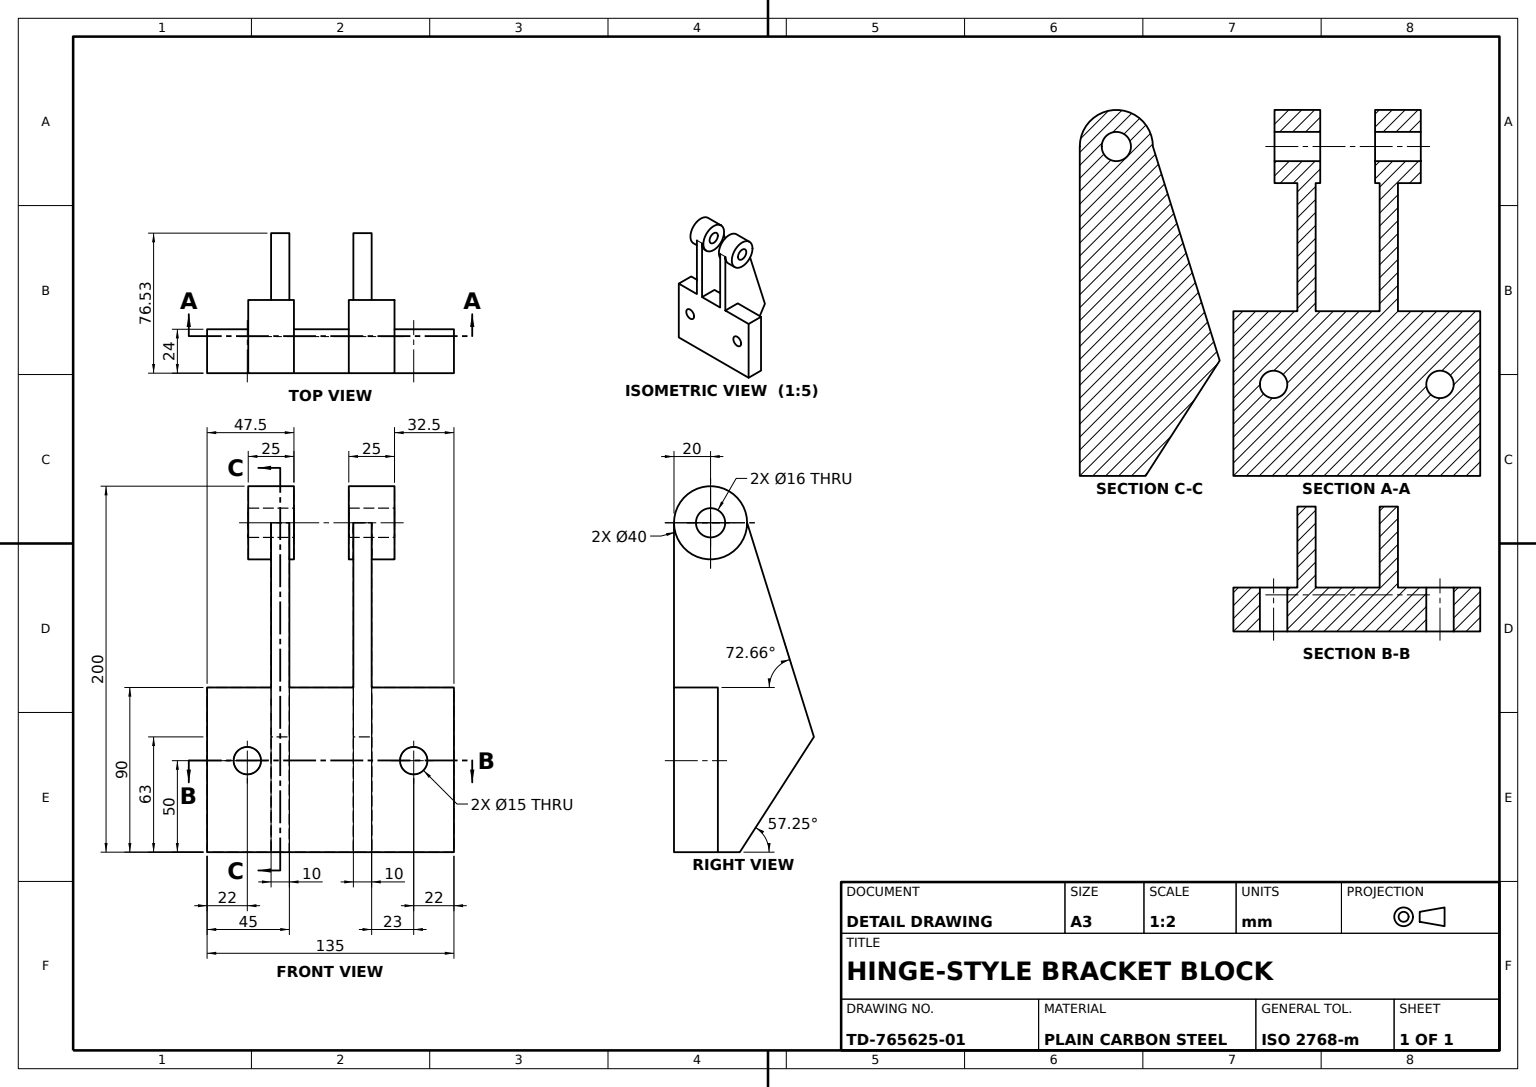
from build123d import *

# Parameters (mm, degrees)
BASE_PLATE_SKETCH_W     = 135
BASE_PLATE_SKETCH_H     = 90
BASE_PLATE_DEPTH        = 24
LUG_1_DEPTH             = 10
LUG_1_BOSS_SKETCH_R     = 20
LUG_1_PIVOT_BOSS_DEPTH  = 12.5
LUG_2_DEPTH             = 10
LUG_2_BOSS_SKETCH_R     = 20
LUG_2_PIVOT_BOSS_DEPTH  = 12.5
PIVOT_HOLE_SKETCH_R     = 8
PIVOT_HOLE_16_DEPTH     = 238.407720253
MOUNTING_HOLES_SKETCH_R = 7.5
MOUNTING_HOLES_2X_DEPTH = 247.94927469


with BuildPart() as part:
    # Base Plate Sketch → Base Plate (new body)
    with BuildSketch(Plane.XY):
        with Locations((67.5, 45)):
            Rectangle(BASE_PLATE_SKETCH_W, BASE_PLATE_SKETCH_H)
    extrude(amount=-BASE_PLATE_DEPTH)

    # Lug 1 Profile → Lug 1 (add)
    with BuildSketch(Plane(origin=(90, 0, 0), x_dir=(0, 0, -1), z_dir=(1, 0, 0))):
        with BuildLine():
            Line((0, 90), (0, 180))
            ThreePointArc((0, 180), (20, 160), (40, 180))
            Line((40, 180), (76.525653448, 63))
            Line((76.525653448, 63), (36, 0))
            Line((36, 0), (24, 0))
            Line((24, 0), (24, 90))
            Line((24, 90), (0, 90))
        make_face()
    extrude(amount=-LUG_1_DEPTH)

    # Lug 1 Boss Sketch → Lug 1 Pivot Boss (add, symmetric)
    with BuildSketch(Plane(origin=(90, 0, 0), x_dir=(0, 0, -1), z_dir=(1, 0, 0))):
        with Locations((20, 180)):
            Circle(LUG_1_BOSS_SKETCH_R)
    extrude(amount=LUG_1_PIVOT_BOSS_DEPTH, both=True)

    # Lug 2 Profile → Lug 2 (add)
    with BuildSketch(Plane.ZY.offset(-45)):
        with BuildLine():
            Line((-24, 0), (-36, 0))
            Line((-36, 0), (-76.525653448, 63))
            Line((-76.525653448, 63), (-40, 180))
            ThreePointArc((-40, 180), (-20, 160), (0, 180))
            Line((0, 180), (0, 90))
            Line((0, 90), (-24, 90))
            Line((-24, 90), (-24, 0))
        make_face()
    extrude(amount=LUG_2_DEPTH)

    # Lug 2 Boss Sketch → Lug 2 Pivot Boss (add, symmetric)
    with BuildSketch(Plane.ZY.offset(-35)):
        with Locations(Location((-20, 180, 0), (0, 0, 180))):
            Circle(LUG_2_BOSS_SKETCH_R)
    extrude(amount=LUG_2_PIVOT_BOSS_DEPTH, both=True)

    # Pivot Hole Sketch → Pivot Hole Ø16 (cut, through all)
    with BuildSketch(Plane(origin=(102.5, 0, 0), x_dir=(0, 0, -1), z_dir=(1, 0, 0))):
        with Locations(Location((20, 180, 0), (0, 0, 180))):
            Circle(PIVOT_HOLE_SKETCH_R)
    extrude(amount=-PIVOT_HOLE_16_DEPTH, mode=Mode.SUBTRACT)

    # Mounting Holes Sketch → Mounting Holes 2x (cut, through all)
    with BuildSketch(Plane(origin=(0, 0, -24), x_dir=(-1, 0, 0), z_dir=(0, 0, -1))):
        with Locations((-113, 50)):
            Circle(MOUNTING_HOLES_SKETCH_R)
        with Locations((-22, 50)):
            Circle(MOUNTING_HOLES_SKETCH_R)
    extrude(amount=-MOUNTING_HOLES_2X_DEPTH, mode=Mode.SUBTRACT)


solid = part.part
